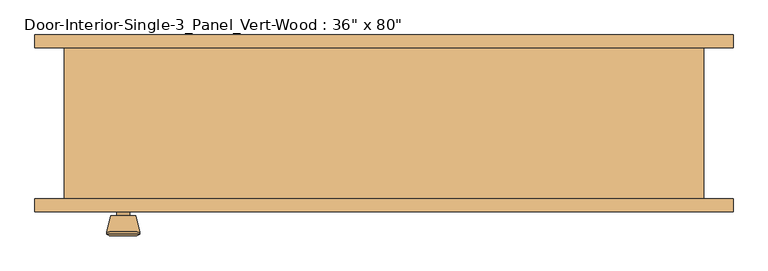
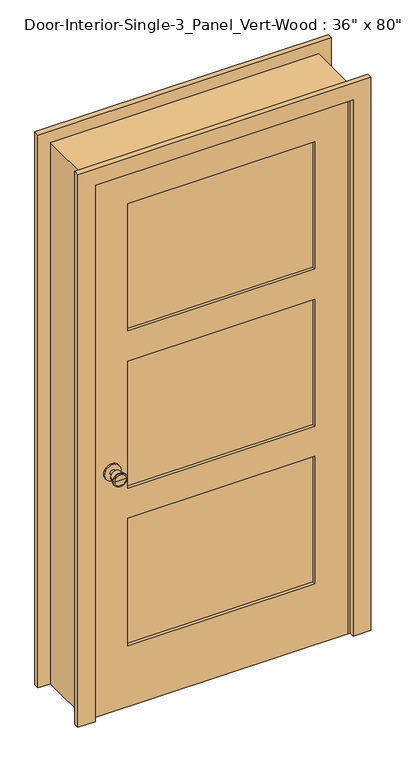
"""IFC4 building model written with IfcOpenShell, lengths in millimetres: door geometry."""

from ifc_helpers import new_model, si_unit, point, frame, frame_2d, origin, place, context, project, spatial, polyline, circle_curve, trimmed, segment, composite_curve, outline, extrude, faceted_brep, source, transform, mapped, element, save
from ifc_brep_helpers import plane_surface, cylinder_surface, revolved_surface, advanced_brep


def door_80766924(model_context):
    return source(origin(), model_context, "Body", "SolidModel", [
        advanced_brep(
        [(-393.7, -70.2, 914.4), (-403.7, -70.2, 914.4), (-383.7, -70.2, 914.4), (-373.2241324, -21.2, 914.4), (-414.1758676, -21.2, 914.4), (-393.7, -21.2, 914.4), (-368.7, -23.0278681, 914.4), (-418.7, -23.0278681, 914.4), (-368.7, -26.4915463, 914.4), (-418.7, -26.4915463, 914.4), (-375.063764, -51.2, 914.4), (-412.336236, -51.2, 914.4), (-383.7, -51.2, 914.4), (-403.7, -51.2, 914.4)],
        [
            (0, 1),
            (1, 2, circle_curve(frame((-393.7, -70.2, 914.4), z_axis=(0.0, -1.0, 0.0), x_axis=(-1.0, 0.0, 0.0)), 10.0)),
            (2, 0),
            (2, 1, circle_curve(frame((-393.7, -70.2, 914.4), z_axis=(0.0, -1.0, 0.0), x_axis=(-1.0, 0.0, 0.0)), 10.0)),
            (3, 4, circle_curve(frame((-393.7, -21.2, 914.4), z_axis=(0.0, 1.0, 0.0), x_axis=(-1.0, 0.0, 0.0)), 20.4758676)),
            (4, 5),
            (5, 3),
            (4, 3, circle_curve(frame((-393.7, -21.2, 914.4), z_axis=(0.0, 1.0, 0.0), x_axis=(-1.0, 0.0, 0.0)), 20.4758676)),
            (6, 7, circle_curve(frame((-393.7, -23.0278681, 914.4), z_axis=(0.0, 1.0, 0.0), x_axis=(-1.0, 0.0, 0.0)), 25.0)),
            (7, 4),
            (3, 6),
            (7, 6, circle_curve(frame((-393.7, -23.0278681, 914.4), z_axis=(0.0, 1.0, 0.0), x_axis=(-1.0, 0.0, 0.0)), 25.0)),
            (8, 9, circle_curve(frame((-393.7, -26.4915463, 914.4), z_axis=(0.0, 1.0, 0.0), x_axis=(-1.0, 0.0, 0.0)), 25.0)),
            (9, 7),
            (6, 8),
            (9, 8, circle_curve(frame((-393.7, -26.4915463, 914.4), z_axis=(0.0, 1.0, 0.0), x_axis=(-1.0, 0.0, 0.0)), 25.0)),
            (10, 11, circle_curve(frame((-393.7, -51.2, 914.4), z_axis=(0.0, 1.0, 0.0), x_axis=(-1.0, 0.0, 0.0)), 18.636236)),
            (11, 9),
            (8, 10),
            (11, 10, circle_curve(frame((-393.7, -51.2, 914.4), z_axis=(0.0, 1.0, 0.0), x_axis=(-1.0, 0.0, 0.0)), 18.636236)),
            (12, 13, circle_curve(frame((-393.7, -51.2, 914.4), z_axis=(0.0, 1.0, 0.0), x_axis=(-1.0, 0.0, 0.0)), 10.0)),
            (13, 11),
            (10, 12),
            (13, 12, circle_curve(frame((-393.7, -51.2, 914.4), z_axis=(0.0, 1.0, 0.0), x_axis=(-1.0, 0.0, 0.0)), 10.0)),
            (1, 13),
            (12, 2),
        ],
        [
            plane_surface(frame((-393.7, -70.2, 914.4), z_axis=(0.0, -1.0, 0.0), x_axis=(-1.0, 0.0, 0.0))),
            plane_surface(frame((-393.7, -21.2, 914.4), z_axis=(0.0, 1.0, 0.0), x_axis=(-1.0, 0.0, 0.0))),
            revolved_surface(polyline([(-414.1758676, -21.2, 914.4), (-418.7, -23.0278681, 914.4)]), (-393.7, -70.2, 914.4), (0.0, -1.0, 0.0)),
            cylinder_surface(frame((-393.7, -70.2, 914.4), z_axis=(0.0, -1.0, 0.0), x_axis=(-1.0, 0.0, 0.0)), 25.0),
            revolved_surface(polyline([(-418.7, -26.4915463, 914.4), (-412.336236, -51.2, 914.4)]), (-393.7, -70.2, 914.4), (0.0, -1.0, 0.0)),
            plane_surface(frame((-393.7, -51.2, 914.4), z_axis=(0.0, -1.0, 0.0), x_axis=(-1.0, 0.0, 0.0))),
            cylinder_surface(frame((-393.7, -70.2, 914.4), z_axis=(0.0, -1.0, 0.0), x_axis=(-1.0, 0.0, 0.0)), 10.0),
        ],
        [
            (0, [[1, 2, 3]]),
            (0, [[-3, 4, -1]]),
            (1, [[5, 6, 7]]),
            (1, [[8, -7, -6]]),
            (2, [[9, 10, -5, 11]]),
            (2, [[12, -11, -8, -10]]),
            (3, [[13, 14, -9, 15]]),
            (3, [[16, -15, -12, -14]]),
            (4, [[17, 18, -13, 19]]),
            (4, [[20, -19, -16, -18]]),
            (5, [[21, 22, -17, 23]]),
            (5, [[24, -23, -20, -22]]),
            (6, [[-2, 25, -21, 26]]),
            (6, [[-4, -26, -24, -25]]),
        ],
    ),
        extrude(outline(composite_curve([segment(trimmed(circle_curve(frame_2d((914.4, -393.7)), 30.0), [point((914.4, -423.7))], [point((914.4, -363.7))], False, "CARTESIAN"), True, "CONTINUOUS"), segment(trimmed(circle_curve(frame_2d((914.4, -393.7)), 30.0), [point((914.4, -363.7))], [point((914.4, -423.7))], False, "CARTESIAN"), True, "CONTINUOUS")], self_intersect=False)), frame((0.0, -76.2, 0.0), z_axis=(0.0, 1.0, 0.0), x_axis=(0.0, 0.0, 1.0)), (0.0, 0.0, 1.0), 6.0),
        advanced_brep(
        [(-393.7, -117.125, 914.4), (-383.7, -117.125, 914.4), (-403.7, -117.125, 914.4), (-373.2241324, -166.125, 914.4), (-393.7, -166.125, 914.4), (-414.1758676, -166.125, 914.4), (-368.7, -164.2971319, 914.4), (-418.7, -164.2971319, 914.4), (-368.7, -160.8334537, 914.4), (-418.7, -160.8334537, 914.4), (-375.063764, -136.125, 914.4), (-412.336236, -136.125, 914.4), (-383.7, -136.125, 914.4), (-403.7, -136.125, 914.4)],
        [
            (0, 1),
            (1, 2, circle_curve(frame((-393.7, -117.125, 914.4), z_axis=(0.0, 1.0, 0.0), x_axis=(-1.0, 0.0, 0.0)), 10.0)),
            (2, 0),
            (2, 1, circle_curve(frame((-393.7, -117.125, 914.4), z_axis=(0.0, 1.0, 0.0), x_axis=(-1.0, 0.0, 0.0)), 10.0)),
            (3, 4),
            (4, 5),
            (5, 3, circle_curve(frame((-393.7, -166.125, 914.4), z_axis=(0.0, -1.0, 0.0), x_axis=(-1.0, 0.0, 0.0)), 20.4758676)),
            (3, 5, circle_curve(frame((-393.7, -166.125, 914.4), z_axis=(0.0, -1.0, 0.0), x_axis=(-1.0, 0.0, 0.0)), 20.4758676)),
            (6, 3),
            (5, 7),
            (7, 6, circle_curve(frame((-393.7, -164.2971319, 914.4), z_axis=(0.0, -1.0, 0.0), x_axis=(-1.0, 0.0, 0.0)), 25.0)),
            (6, 7, circle_curve(frame((-393.7, -164.2971319, 914.4), z_axis=(0.0, -1.0, 0.0), x_axis=(-1.0, 0.0, 0.0)), 25.0)),
            (8, 6),
            (7, 9),
            (9, 8, circle_curve(frame((-393.7, -160.8334537, 914.4), z_axis=(0.0, -1.0, 0.0), x_axis=(-1.0, 0.0, 0.0)), 25.0)),
            (8, 9, circle_curve(frame((-393.7, -160.8334537, 914.4), z_axis=(0.0, -1.0, 0.0), x_axis=(-1.0, 0.0, 0.0)), 25.0)),
            (10, 8),
            (9, 11),
            (11, 10, circle_curve(frame((-393.7, -136.125, 914.4), z_axis=(0.0, -1.0, 0.0), x_axis=(-1.0, 0.0, 0.0)), 18.636236)),
            (10, 11, circle_curve(frame((-393.7, -136.125, 914.4), z_axis=(0.0, -1.0, 0.0), x_axis=(-1.0, 0.0, 0.0)), 18.636236)),
            (12, 10),
            (11, 13),
            (13, 12, circle_curve(frame((-393.7, -136.125, 914.4), z_axis=(0.0, -1.0, 0.0), x_axis=(-1.0, 0.0, 0.0)), 10.0)),
            (12, 13, circle_curve(frame((-393.7, -136.125, 914.4), z_axis=(0.0, -1.0, 0.0), x_axis=(-1.0, 0.0, 0.0)), 10.0)),
            (1, 12),
            (13, 2),
        ],
        [
            plane_surface(frame((-393.7, -117.125, 914.4), z_axis=(0.0, 1.0, 0.0), x_axis=(-1.0, 0.0, 0.0))),
            plane_surface(frame((-393.7, -166.125, 914.4), z_axis=(0.0, -1.0, 0.0), x_axis=(-1.0, 0.0, 0.0))),
            revolved_surface(polyline([(-414.1758676, -166.125, 914.4), (-418.7, -164.2971319, 914.4)]), (-393.7, -117.125, 914.4), (0.0, 1.0, 0.0)),
            cylinder_surface(frame((-393.7, -117.125, 914.4), z_axis=(0.0, 1.0, 0.0), x_axis=(-1.0, 0.0, 0.0)), 25.0),
            revolved_surface(polyline([(-418.7, -160.8334537, 914.4), (-412.336236, -136.125, 914.4)]), (-393.7, -117.125, 914.4), (0.0, 1.0, 0.0)),
            plane_surface(frame((-393.7, -136.125, 914.4), z_axis=(0.0, 1.0, 0.0), x_axis=(-1.0, 0.0, 0.0))),
            cylinder_surface(frame((-393.7, -117.125, 914.4), z_axis=(0.0, 1.0, 0.0), x_axis=(-1.0, 0.0, 0.0)), 10.0),
        ],
        [
            (0, [[1, 2, 3]]),
            (0, [[-3, 4, -1]]),
            (1, [[5, 6, 7]]),
            (1, [[-6, -5, 8]]),
            (2, [[9, -7, 10, 11]]),
            (2, [[-10, -8, -9, 12]]),
            (3, [[13, -11, 14, 15]]),
            (3, [[-14, -12, -13, 16]]),
            (4, [[17, -15, 18, 19]]),
            (4, [[-18, -16, -17, 20]]),
            (5, [[21, -19, 22, 23]]),
            (5, [[-22, -20, -21, 24]]),
            (6, [[25, -23, 26, -2]]),
            (6, [[-26, -24, -25, -4]]),
        ],
    ),
        extrude(outline(composite_curve([segment(trimmed(circle_curve(frame_2d((914.4, -393.7)), 30.0), [point((914.4, -423.7))], [point((914.4, -363.7))], False, "CARTESIAN"), True, "CONTINUOUS"), segment(trimmed(circle_curve(frame_2d((914.4, -393.7)), 30.0), [point((914.4, -363.7))], [point((914.4, -423.7))], False, "CARTESIAN"), True, "CONTINUOUS")], self_intersect=False)), frame((0.0, -117.125, 0.0), z_axis=(0.0, 1.0, 0.0), x_axis=(0.0, 0.0, 1.0)), (0.0, 0.0, 1.0), 6.0),
        faceted_brep([(482.6, -111.125, 0.0), (457.2, -111.125, 0.0), (457.2, -76.2, 0.0), (444.5, -76.2, 0.0), (444.5, -41.275, 0.0), (457.2, -41.275, 0.0), (457.2, 117.475, 0.0), (482.6, 117.475, 0.0), (482.6, 117.475, 2057.4), (482.6, -111.125, 2057.4), (457.2, 117.475, 2032.0), (-457.2, 117.475, 2032.0), (-457.2, 117.475, 0.0), (-482.6, 117.475, 0.0), (-482.6, 117.475, 2057.4), (457.2, -41.275, 2032.0), (444.5, -41.275, 2019.3), (-444.5, -41.275, 2019.3), (-444.5, -41.275, 0.0), (-457.2, -41.275, 0.0), (-457.2, -41.275, 2032.0), (444.5, -76.2, 2019.3), (457.2, -76.2, 2032.0), (-457.2, -76.2, 2032.0), (-457.2, -76.2, 0.0), (-444.5, -76.2, 0.0), (-444.5, -76.2, 2019.3), (457.2, -111.125, 2032.0), (-482.6, -111.125, 2057.4), (-482.6, -111.125, 0.0), (-457.2, -111.125, 0.0), (-457.2, -111.125, 2032.0)], [[[0, 1, 2, 3, 4, 5, 6, 7]], [[7, 8, 9, 0]], [[6, 10, 11, 12, 13, 14, 8, 7]], [[5, 15, 10, 6]], [[4, 16, 17, 18, 19, 20, 15, 5]], [[3, 21, 16, 4]], [[2, 22, 23, 24, 25, 26, 21, 3]], [[1, 27, 22, 2]], [[0, 9, 28, 29, 30, 31, 27, 1]], [[8, 14, 28, 9]], [[15, 20, 11, 10]], [[21, 26, 17, 16]], [[27, 31, 23, 22]], [[29, 13, 12, 19, 18, 25, 24, 30]], [[14, 13, 29, 28]], [[20, 19, 12, 11]], [[26, 25, 18, 17]], [[31, 30, 24, 23]]]),
        extrude(outline(polyline([(2032.0, -457.2), (0.0, -457.2), (0.0, 457.2), (2032.0, 457.2), (2032.0, -457.2)]), holes=[polyline([(1912.9375, -336.55), (1912.9375, 336.55), (1428.75, 336.55), (1428.75, -336.55), (1912.9375, -336.55)]), polyline([(715.9625, -336.55), (715.9625, 336.55), (231.775, 336.55), (231.775, -336.55), (715.9625, -336.55)]), polyline([(1314.45, -336.55), (1314.45, 336.55), (830.2625, 336.55), (830.2625, -336.55), (1314.45, -336.55)])]), frame((0.0, -111.125, 0.0), z_axis=(0.0, 1.0, 0.0), x_axis=(0.0, 0.0, 1.0)), (0.0, 0.0, 1.0), 34.925),
        extrude(outline(polyline([(336.55, -87.8416667), (336.55, -99.4833333), (-336.55, -99.4833333), (-336.55, -87.8416667), (336.55, -87.8416667)])), frame((0.0, 0.0, 1428.75), z_axis=(0.0, 0.0, 1.0), x_axis=(1.0, 0.0, 0.0)), (0.0, 0.0, 1.0), 484.1875),
        extrude(outline(polyline([(336.55, -87.8416667), (336.55, -99.4833333), (-336.55, -99.4833333), (-336.55, -87.8416667), (336.55, -87.8416667)])), frame((0.0, 0.0, 231.775), z_axis=(0.0, 0.0, 1.0), x_axis=(1.0, 0.0, 0.0)), (0.0, 0.0, 1.0), 484.1875),
        extrude(outline(polyline([(336.55, -87.8416667), (336.55, -99.4833333), (-336.55, -99.4833333), (-336.55, -87.8416667), (336.55, -87.8416667)])), frame((0.0, 0.0, 830.2625), z_axis=(0.0, 0.0, 1.0), x_axis=(1.0, 0.0, 0.0)), (0.0, 0.0, 1.0), 484.1875),
        extrude(outline(polyline([(0.0, 527.05), (2101.85, 527.05), (2101.85, -527.05), (0.0, -527.05), (0.0, -463.55), (2038.35, -463.55), (2038.35, 463.55), (0.0, 463.55), (0.0, 527.05)])), frame((0.0, -130.175, 0.0), z_axis=(0.0, 1.0, 0.0), x_axis=(0.0, 0.0, 1.0)), (0.0, 0.0, 1.0), 19.05),
        extrude(outline(polyline([(0.0, 527.05), (2101.85, 527.05), (2101.85, -527.05), (0.0, -527.05), (0.0, -463.55), (2038.35, -463.55), (2038.35, 463.55), (0.0, 463.55), (0.0, 527.05)])), frame((0.0, 117.475, 0.0), z_axis=(0.0, 1.0, 0.0), x_axis=(0.0, 0.0, 1.0)), (0.0, 0.0, 1.0), 19.05),
    ])


if __name__ == "__main__":
    model = new_model("IFC4")
    model_context = context("Model", 3, world=origin())
    ifc_project = project(units=[si_unit("LENGTHUNIT", "METRE", prefix="MILLI")], contexts=[model_context])
    site = spatial("IfcSite", under=ifc_project)
    building = spatial("IfcBuilding", under=site)
    placement = place(None, origin())
    door_shape = door_80766924(model_context)
    element("IfcDoor", 1, ObjectType="Door-Interior-Single-3_Panel_Vert-Wood : 36\" x 80\"", at=placement, inside=building, context=model_context, shape_type="MappedRepresentation", body=[
        mapped(door_shape, transform((0.0, 0.0, 0.0), x_axis=(1.0, 0.0, 0.0), y_axis=(0.0, 1.0, 0.0), z_axis=(0.0, 0.0, 1.0))),
    ])
    save(model, "model.ifc")

# Revit data of these elements
# Type "Door-Interior-Single-3_Panel_Vert-Wood : 36\" x 80\""
#   Type Mark = "10"
#   Assembly Code = "C1020300"
#   Analytic Construction = "Wooden"
#   Top Rail = 0' - 4 11/16"
#   Thickness = 0' - 1 3/8"
#   Thermal Resistance (R) = 2.5876 (h·ft²·°F)/BTU
#   Swing Angle [instance default] = 90.00°
#   Stiles = 0' - 4 3/4"
#   Rough Width = 3' - 2"
#   Rough Height = 6' - 9"
#   Intermediate Rail = 0' - 4 1/2"
#   Height = 6' - 8"
#   Width = 3' - 0"
#   Heat Transfer Coefficient (U) = 0.3865 BTU/(h·ft²·°F)
#   Bottom Rail = 0' - 9 1/8"
#   Trim Material = Cherry
#   Panel Material = Cherry
#   Frame Material = Cherry
#   Door Handle Material = Aluminum
#   Visual Light Transmittance = 0
#   Solar Heat Gain Coefficient = 0
#   Wall Closure = (empty or 0)
#   Function = (empty or 0)
# Element 1 (IfcDoor, "Door-Interior-Single-3_Panel_Vert-Wood : 36\" x 80\"")
#   Materials on its faces: "Cherry", "Aluminum"
# Materials
#   "Cherry": class "Wood", colour RGB 226 177 128, transparency 0, Description = "Prunus Serotina", Cost = 0
#   "Aluminum": class "Metal", colour RGB 247 247 247, transparency 0, Description = "Aluminum 6061", Cost = 0
